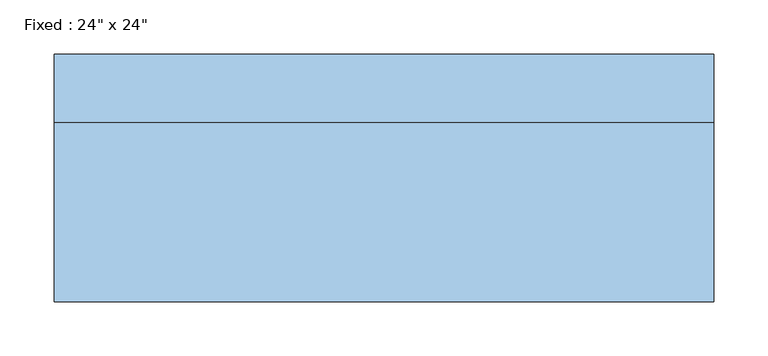
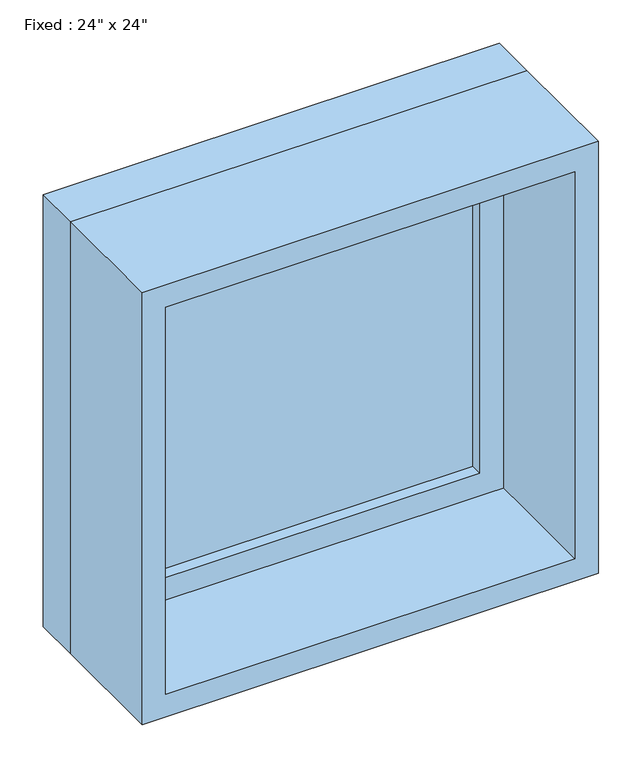
"""IFC4 building model written with IfcOpenShell, lengths in millimetres: window geometry."""

from ifc_helpers import new_model, si_unit, frame, origin, place, context, project, spatial, polyline, outline, extrude, source, transform, mapped, element, save


def window_80340324(model_context):
    return source(origin(), model_context, "Body", "SweptSolid", [
        extrude(outline(polyline([(203.2, 66.675), (-279.4, 66.675), (-279.4, 79.375), (203.2, 79.375), (203.2, 66.675)])), frame((0.0, 0.0, 977.9), z_axis=(0.0, 0.0, 1.0), x_axis=(1.0, 0.0, 0.0)), (0.0, 0.0, 1.0), 482.6),
        extrude(outline(polyline([(1504.95, -323.85), (933.45, -323.85), (933.45, 247.65), (1504.95, 247.65), (1504.95, -323.85)]), holes=[polyline([(1460.5, -279.4), (1460.5, 203.2), (977.9, 203.2), (977.9, -279.4), (1460.5, -279.4)])]), frame((0.0, 50.8, 0.0), z_axis=(0.0, 1.0, 0.0), x_axis=(0.0, 0.0, 1.0)), (0.0, 0.0, 1.0), 44.45),
        extrude(outline(polyline([(1524.0, -342.9), (914.4, -342.9), (914.4, 266.7), (1524.0, 266.7), (1524.0, -342.9)]), holes=[polyline([(1492.25, -311.15), (1492.25, 234.95), (946.15, 234.95), (946.15, -311.15), (1492.25, -311.15)])]), frame((0.0, -114.3, 0.0), z_axis=(0.0, 1.0, 0.0), x_axis=(0.0, 0.0, 1.0)), (0.0, 0.0, 1.0), 165.1),
        extrude(outline(polyline([(1524.0, 266.7), (1524.0, -342.9), (914.4, -342.9), (914.4, 266.7), (1524.0, 266.7)]), holes=[polyline([(1504.95, 247.65), (933.45, 247.65), (933.45, -323.85), (1504.95, -323.85), (1504.95, 247.65)])]), frame((0.0, 50.8, 0.0), z_axis=(0.0, 1.0, 0.0), x_axis=(0.0, 0.0, 1.0)), (0.0, 0.0, 1.0), 63.5),
    ])


if __name__ == "__main__":
    model = new_model("IFC4")
    model_context = context("Model", 3, world=origin())
    ifc_project = project(units=[si_unit("LENGTHUNIT", "METRE", prefix="MILLI")], contexts=[model_context])
    site = spatial("IfcSite", under=ifc_project)
    building = spatial("IfcBuilding", under=site)
    placement = place(None, origin())
    window_shape = window_80340324(model_context)
    element("IfcWindow", 1, ObjectType="Fixed : 24\" x 24\"", at=placement, inside=building, context=model_context, shape_type="MappedRepresentation", body=[
        mapped(window_shape, transform((0.0, 0.0, 0.0), x_axis=(1.0, 0.0, 0.0), y_axis=(0.0, 1.0, 0.0), z_axis=(0.0, 0.0, 1.0))),
    ])
    save(model, "model.ifc")

# Revit data of these elements
# Type "Fixed : 24\" x 24\""
#   Type Mark = "4"
#   Construction Type Id = "GSP4R"
#   Assembly Code = "B2020100"
#   Analytic Construction = "1/8 in Pilkington single glazing"
#   Visual Light Transmittance = 0.9
#   Solar Heat Gain Coefficient = 0.78
#   Heat Transfer Coefficient (U) = 0.6496 BTU/(h·ft²·°F)
#   Height = 2' - 0"
#   Default Sill Height = 3' - 0"
#   Width = 2' - 0"
#   Window Inset = 0' - 0 3/4"
#   Define Thermal Properties by = 1
#   Define Thermal Properties by = 1
#   Glass Pane Material = Glass
#   Sash Material = Sash
#   Wall Closure = (empty or 0)
# Element 1 (IfcWindow, "Fixed : 24\" x 24\"")
#   Materials on its faces: "Sash", "Glass"
# Materials
#   "Glass": class "Glass", colour RGB 0 128 192, transparency 0.75, Description = "Soda Lime Glass", Cost = 0
#   "Sash": class "Wood", colour RGB 224 178 126, transparency 0, Cost = 0
